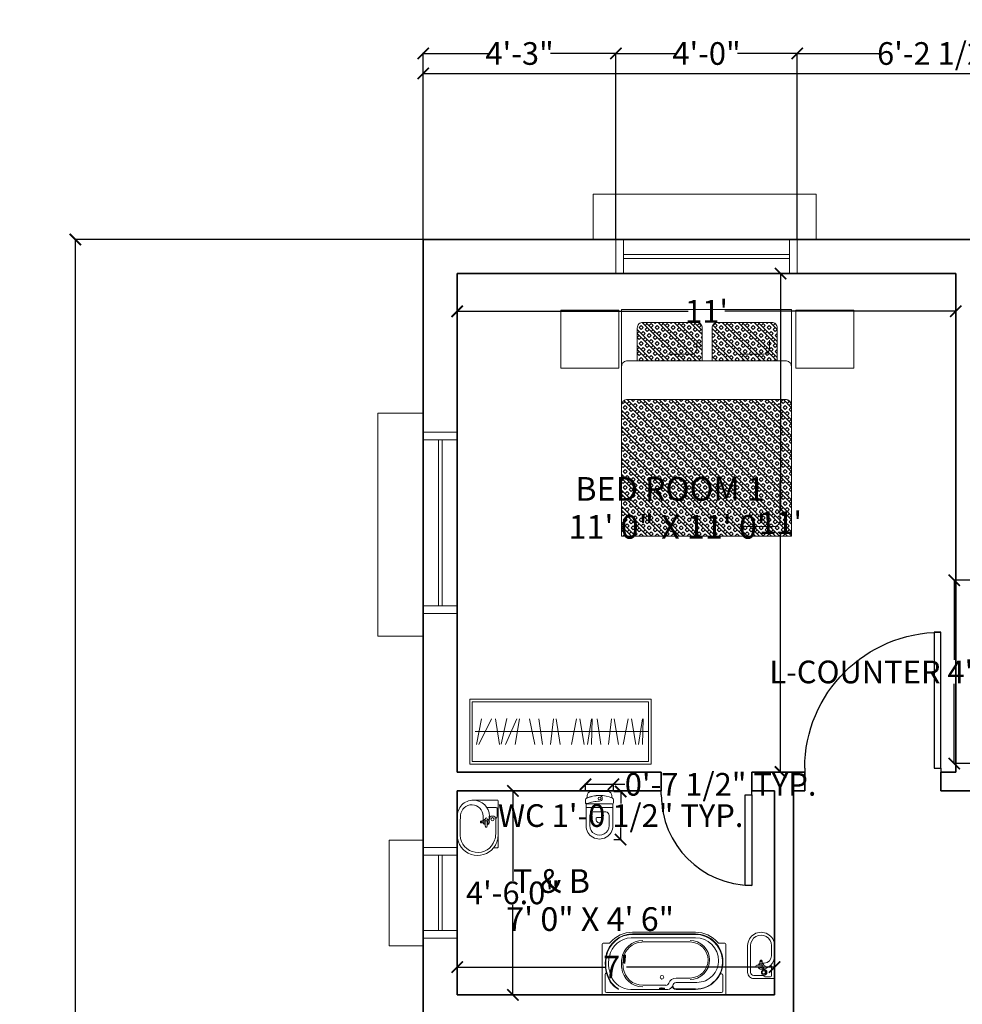
# Model space of a CAD drawing. Units: inches. Extents: x 844 to 2234, y 346 to 1084.
# Tile 3 of 93: x 844 to 1093, y 823 to 1084. Entities that reach past the tile are written whole.
import ezdxf

# ---------------------------------------------------------------- set-up
doc = ezdxf.new("R2010")
doc.units = ezdxf.units.IN
doc.header["$MEASUREMENT"] = 0
for name, color, linetype, lineweight in [('A-ANNO-DIMS', 2, 'Continuous', 18), ('A-AREA-IDEN', 7, 'Continuous', 18), ('A-FLOR-FIXT', 8, 'Continuous', 18), ('A-WALL', 7, 'Continuous', 35), ('beds', 130, 'Continuous', 18), ('doors', 170, 'Continuous', 25), ('furniture', 8, 'Continuous', 18), ('windows', 1, 'Continuous', 18)]:
    doc.layers.add(name, color=color, linetype=linetype, lineweight=lineweight)
doc.styles.get("Standard").update_dxf_attribs({"font": 'arial.ttf'})
doc.dimstyles.get("Standard").update_dxf_attribs({"dimtxt": 6, "dimasz": 3, "dimexe": 0.18, "dimexo": 0.0625, "dimgap": 0.09, "dimtad": 0, "dimtih": 1, "dimtoh": 1, "dimdec": 1, "dimzin": 0, "dimdsep": 46, "dimlunit": 3, "dimtxsty": 'Standard', "dimblk": 'ARCHTICK', "dimcen": 0.09, "dimadec": 0, "dimazin": 0, "dimtfac": 1, "dimtdec": 1, "dimtofl": 0, "dimtmove": 0, "dimatfit": 3, "dimfxl": 1, "dimtolj": 1, "dimtzin": 0, "dimarcsym": 0})
pattern_1 = [(135, (-1377.70473, -125.71507), (-0.070710678, -0.070710678), []), (135, (-1377.68705, -125.69739), (-0.070710678, -0.070710678), []), (45, (-1377.70473, -125.71507), (-0.070710678, 0.070710678), [-0.025, 0.025]), (45, (-1377.72241, -125.69739), (-0.070710678, 0.070710678), [-0.025, 0.025]), (45, (-1377.74009, -125.67972), (-0.070710678, 0.070710678), [0.025, -0.025]), (45, (-1377.75776, -125.66204), (-0.070710678, 0.070710678), [0.025, -0.025]), (135, (-1377.66938, -125.67972), (-0.070710678, -0.070710678), [0.025, -0.025]), (135, (-1377.6517, -125.66204), (-0.070710678, -0.070710678), [0.025, -0.025])]

# ---------------------------------------------------------------- blocks, each defined once
blk = doc.blocks.new('*U2')
for p, q in [((0, 0), (0, -6)), ((36, 0), (36, -6))]:
    blk.add_line(p, q)
blk.add_lwpolyline([(0, 0), (0, 36), (1.75, 36), (1.75, 0)], close=True)
blk.add_arc((0, 0), 36, 0, 90)
blk = doc.blocks.new('*U4')
for p, q in [((0, 0), (0, -6)), ((24, 0), (24, -6))]:
    blk.add_line(p, q)
blk.add_lwpolyline([(0, 0), (0, 24), (1.75, 24), (1.75, 0)], close=True)
blk.add_arc((0, 0), 24, 0, 90)
blk = doc.blocks.new('MAT-P10')
h = blk.add_hatch()
h.set_pattern_fill('BOX', color=256, scale=0.1, angle=45, style=0)
h.set_pattern_definition(pattern_1)
h.paths.add_polyline_path([(-0.1565, 1.4605), (0.417, 1.4605), (0.417, 1.7513, 0.414214), (0.367, 1.8013), (-0.1065, 1.8013, 0.414214), (-0.1565, 1.7513)])
h.paths.add_polyline_path([(0.5052, 1.4604), (1.0792, 1.4604), (1.0792, 1.7513, 0.414214), (1.0292, 1.8013), (0.5552, 1.8013, 0.414214), (0.5052, 1.7513)])
h = blk.add_hatch()
h.set_pattern_fill('BOX', color=256, scale=0.1, angle=45, style=0)
h.set_pattern_definition(pattern_1)
edge = h.paths.add_edge_path()
edge.add_line((1.2049, -0.085), (1.2049, 1.0625))
edge.add_ellipse((1.1608, 1.0627), major_axis=(0, 0.0568), ratio=0.776379, start_angle=270, end_angle=360)
edge.add_line((1.1608, 1.1195), (-0.251, 1.1195))
edge.add_ellipse((-0.251, 1.0627), major_axis=(0, 0.0568), ratio=0.776379, start_angle=0, end_angle=88.13958)
edge.add_line((-0.2951, 1.0641), (-0.2951, -0.085))
edge.add_line((-0.2951, -0.085), (1.2049, -0.085))
for p, q in [((-0.251, 1.4605), (1.1608, 1.4604)), ((-0.251, 1.1195), (1.1608, 1.1195)), ((1.1017, 0.406), (1.1017, 0.0572)), ((1.0576, 0.0004), (0.7754, 0.0004))]:
    blk.add_line(p, q)
for points in [[(1.2049, -0.085), (-0.2951, -0.085), (-0.2951, 1.9151), (1.2049, 1.915)], [(-0.8301, 1.9091), (-0.3191, 1.9091), (-0.3191, 1.3981), (-0.8301, 1.3981)], [(1.2441, 1.9091), (1.755, 1.9091), (1.755, 1.3981), (1.2441, 1.3981)]]:
    blk.add_lwpolyline(points, close=True)
for points in [[(0.417, 1.4604), (0.417, 1.7513, 0.414214), (0.367, 1.8013), (-0.1065, 1.8013, 0.414214), (-0.1565, 1.7513), (-0.1565, 1.4604)], [(1.0792, 1.4603), (1.0792, 1.7513, 0.414214), (1.0292, 1.8013), (0.5552, 1.8013, 0.414214), (0.5052, 1.7513), (0.5052, 1.4604)], [(0.3702, 1.6242), (0.3702, 1.5715, -0.414214), (0.3202, 1.5215), (0.1113, 1.5215)], [(1.0117, 1.6438), (1.0117, 1.5715, -0.414214), (0.9617, 1.5215), (0.7528, 1.5215)]]:
    blk.add_lwpolyline(points, format="xyb")
at = {"extrusion": (0, 0, -1)}
for centre, start_param, end_param in [((-0.251, 1.4036), 4.712389, 6.283185), ((1.1608, 1.4036), 0, 1.570796), ((-0.251, 1.0627), 4.712389, 6.283185), ((1.1608, 1.0627), 0, 1.570796), ((1.0576, 0.0572), 1.570796, 3.141593), ((1.0576, 0.0572), 1.570796, 3.141593)]:
    blk.add_ellipse(centre, major_axis=(0, 0.0568), ratio=0.776379, start_param=start_param, end_param=end_param, dxfattribs=at)
blk = doc.blocks.new('A$C7A17768A')
for p, q in [((-2.8, 0), (0, 0)), ((-2.8, -1), (-2.8, 0)), ((0, -1), (0, 0)), ((-2.76, -0.04), (-0.04, -0.04)), ((-2.76, -0.96), (-2.76, -0.04)), ((-0.04, -0.96), (-0.04, -0.04)), ((-2.617, -0.3), (-2.694, -0.7)), ((-2.66, -0.7), (-2.466, -0.3)), ((-2.403, -0.3), (-2.342, -0.7)), ((-2.229, -0.296), (-2.317, -0.696)), ((-2.074, -0.3), (-2.25, -0.7)), ((-2.096, -0.7), (-2.033, -0.3)), ((-1.875, -0.3), (-1.796, -0.7)), ((-1.732, -0.3), (-1.675, -0.7)), ((-1.555, -0.7), (-1.507, -0.3)), ((-1.467, -0.3), (-1.403, -0.7)), ((-1.227, -0.7), (-1.151, -0.3)), ((-1.098, -0.3), (-1.034, -0.7)), ((-0.98, -0.7), (-0.921, -0.3)), ((-0.908, -0.3), (-0.919, -0.7)), ((-0.834, -0.3), (-0.777, -0.7)), ((-0.657, -0.7), (-0.61, -0.3)), ((-0.57, -0.3), (-0.505, -0.7)), ((-0.429, -0.7), (-0.353, -0.3)), ((-0.301, -0.3), (-0.237, -0.7)), ((-0.192, -0.7), (-0.133, -0.3)), ((-0.12, -0.3), (-0.131, -0.7)), ((-0.04, -0.5), (-2.716, -0.5)), ((-2.8, -1), (0, -1)), ((-2.76, -0.96), (-0.04, -0.96))]:
    blk.add_line(p, q)
blk = doc.blocks.new('2SABICO')
at = {"color": 0, "linetype": 'ByBlock'}
for p, q in [((0.478, 0.195), (0.089, 0.195)), ((0.478, 0.152), (0.089, 0.152)), ((0, 0.106), (0, 0)), ((0, 0), (0, -0.18)), ((0.043, -0.039), (0.043, 0.106)), ((0.135, 0), (0.135, -0.003)), ((0.168, 0.064), (0.168, -0.015)), ((0.192, 0.064), (0.192, -0.015)), ((0.221, 0.012), (0.222, 0.012)), ((0.223, 0.016), (0.223, -0.016)), ((0.224, 0.017), (0.245, 0.017)), ((0.246, 0.016), (0.246, -0.016)), ((0.25, 0.014), (0.246, 0.014)), ((0.26, 0.01), (0.268, 0.01)), ((0.268, -0.01), (0.268, 0.01)), ((0.268, 0.01), (0.269, 0.009)), ((0.269, -0.009), (0.269, 0.009)), ((0.023, -0.057), (0.023, -0.135)), ((0.135, 0), (0.135, -0.039)), ((0.168, -0.015), (0.192, -0.015)), ((0.168, -0.015), (0.168, -0.046)), ((0.192, -0.015), (0.192, -0.046)), ((0.221, -0.012), (0.222, -0.012)), ((0.224, -0.017), (0.245, -0.017)), ((0.225, -0.017), (0.225, -0.047)), ((0.25, -0.014), (0.246, -0.014)), ((0.26, -0.01), (0.268, -0.01)), ((0.268, -0.01), (0.269, -0.009)), ((0.015, -0.195), (0.478, -0.195)), ((0.038, -0.15), (0.179, -0.15)), ((0.33, -0.152), (0.478, -0.152))]:
    blk.add_line(p, q, dxfattribs=at)
for radius in [0.035, 0.023]:
    blk.add_circle((0.089, -0.039), radius, dxfattribs=at)
for centre, radius, start, end in [((0.089, 0.106), 0.089, 90, 180), ((0.089, 0.106), 0.046, 90, 180), ((0.478, 0), 0.195, 270, 90), ((0.478, 0), 0.152, 270, 90), ((0.18, 0), 0.045, 105.6643, 180), ((0.18, 0), 0.042, 106.8152, 252.6853), ((0.18, 0), 0.0235, 121.1327, 237.8651), ((0.18, 0.064), 0.0121, 0, 180), ((0.18, 0), 0.045, 17.0576, 74.3357), ((0.18, 0), 0.042, 287.3147, 73.1848), ((0.18, 0), 0.0235, 302.1349, 58.8673), ((0.221, 0.013), 0.001, 197.9471, 270), ((0.222, 0.013), 0.001, 270, 0), ((0.224, 0.016), 0.001, 90, 180), ((0.245, 0.016), 0.001, 0, 90), ((0.25, 0), 0.0143, 270, 90), ((0.041, -0.057), 0.018, 99.5941, 180), ((0.038, -0.135), 0.015, 180, 270), ((0.037, -0.033), 0.006, 279.5941, 0), ((0.089, -0.039), 0.046, 180, 360), ((0.326, -0.003), 0.191, 180, 270), ((0.18, -0.046), 0.0125, 180, 0), ((0.179, -0.14), 0.01, 270, 42.9682), ((0.221, -0.013), 0.001, 90, 162.0529), ((0.222, -0.013), 0.001, 0, 90), ((0.224, -0.016), 0.001, 180, 270), ((0.33, -0.047), 0.105, 180, 270), ((0.245, -0.016), 0.001, 270, 0), ((0.015, -0.18), 0.015, 180, 270)]:
    blk.add_arc(centre, radius, start, end, dxfattribs=at)
blk = doc.blocks.new('2SAINCO')
at = {"color": 0, "linetype": 'ByBlock'}
for p, q in [((0.06, 0.181), (0.085, 0.181)), ((0.114, 0.203), (0.165, 0.203)), ((0.496, 0.195), (0.178, 0.195)), ((0.18, -0.188), (0.18, 0.188)), ((0.231, 0.185), (0.231, -0.185)), ((0.234, 0.185), (0.234, -0.185)), ((0, -0.121), (0, 0.121)), ((0.496, 0.14), (0.347, 0.14)), ((0.394, 0.05), (0.407, 0.05)), ((0.496, -0.14), (0.347, -0.14)), ((0.394, -0.05), (0.407, -0.05)), ((0.06, -0.181), (0.085, -0.181)), ((0.114, -0.201), (0.165, -0.201)), ((0.114, -0.203), (0.165, -0.203)), ((0.496, -0.195), (0.178, -0.195))]:
    blk.add_line(p, q, dxfattribs=at)
blk.add_circle((0.1, 0), 0.02, dxfattribs=at)
for centre, radius, start, end in [((0.06, 0.121), 0.06, 90, 180), ((0.517, 0), 0.46, 155.909, 204.091), ((0.085, 0.196), 0.015, 270, 344.534), ((0.114, 0.188), 0.015, 90, 164.534), ((0.165, 0.188), 0.015, 0, 90), ((0.221, 0.185), 0.01, 0, 90), ((0.224, 0.185), 0.01, 0, 90), ((0.496, 0), 0.195, 270, 90), ((0.1, 0), 0.0405, 360, 180), ((0.517, 0), 0.458, 180, 204.67), ((0.66, 0.008), 0.52, 180.891, 201.3823), ((2.295, 0), 2, 177.3546, 182.6454), ((0.347, 0.09), 0.05, 90, 177.3546), ((0.677, 0), 0.3, 172.9459, 187.0541), ((0.394, 0.035), 0.015, 90, 172.9459), ((0.407, 0), 0.05, 270, 90), ((0.496, 0), 0.14, 270, 90), ((0.06, -0.121), 0.06, 180, 270), ((0.347, -0.09), 0.05, 182.6454, 270), ((0.394, -0.035), 0.015, 187.0541, 270), ((0.085, -0.196), 0.015, 15.466, 90), ((0.114, -0.188), 0.015, 195.466, 270), ((0.114, -0.188), 0.013, 195.466, 270), ((0.165, -0.188), 0.013, 270, 30), ((0.165, -0.188), 0.015, 270, 0), ((0.221, -0.185), 0.01, 270, 0), ((0.224, -0.185), 0.01, 270, 0)]:
    blk.add_arc(centre, radius, start, end, dxfattribs=at)
blk = doc.blocks.new('2SABACO')
at = {"color": 0}
for p, q in [((1.341, 0.91), (0.429, 0.91)), ((1.341, 0.885), (0.429, 0.885)), ((1.341, 0.879), (0.429, 0.879)), ((-0.015, 0.735), (-0.015, 0.015)), ((0, 0.75), (0.08, 0.75)), ((1.341, 0.831), (0.407, 0.831)), ((1.263, 0.769), (0.562, 0.769)), ((1.77, 0.75), (1.69, 0.75)), ((1.785, 0.015), (1.785, 0.735)), ((0.03, 0.302), (0.03, 0.053)), ((1.263, 0.245), (1.06, 0.245)), ((1.363, 0.181), (1.06, 0.181)), ((1.74, 0.053), (1.74, 0.286)), ((0, 0), (1.77, 0)), ((0.048, 0.035), (1.722, 0.035)), ((0.401, 0.08), (0.942, 0.08)), ((0.578, 0.139), (0.911, 0.139)), ((1.343, 0.086), (1.06, 0.086)), ((1.343, 0.079), (1.06, 0.079))]:
    blk.add_line(p, q, dxfattribs=at)
blk.add_circle((0.855, 0.256), 0.026, dxfattribs=at)
for centre, radius, start, end in [((0.428, 0.49), 0.395, 98.9726, 181.1954), ((0.428, 0.49), 0.389, 98.9726, 181.2301), ((0.429, 0.48), 0.43, 90, 139.2943), ((0.429, 0.48), 0.405, 90, 98.9726), ((0.429, 0.48), 0.399, 90, 98.9726), ((1.341, 0.48), 0.43, 40.7057, 90), ((1.341, 0.485), 0.401, 359.4627, 90), ((1.341, 0.485), 0.394, 3.5237, 90), ((0, 0.735), 0.015, 90, 180), ((0.08, 0.78), 0.03, 270, 319.2943), ((0.425, 0.49), 0.342, 93.1008, 168.0202), ((0.578, 0.481), 0.311, 90, 172.609), ((0.578, 0.481), 0.288, 93.3767, 172.609), ((1.263, 0.507), 0.285, 270, 90), ((1.263, 0.507), 0.262, 270, 90), ((1.341, 0.495), 0.336, 0, 90), ((1.69, 0.78), 0.03, 220.7057, 270), ((1.77, 0.735), 0.015, 0, 90), ((0.559, 0.454), 0.48, 163.1286, 202.3619), ((0.559, 0.454), 0.528, 177.0415, 202.3619), ((0.559, 0.454), 0.521, 177.0156, 202.3619), ((0.79, 0.454), 0.525, 172.609, 180), ((0.79, 0.454), 0.525, 180, 187.391), ((0.79, 0.454), 0.502, 172.609, 180), ((0.79, 0.454), 0.502, 180, 187.391), ((1.343, 0.477), 0.392, 270, 4.5675), ((1.343, 0.477), 0.398, 270, 0.539), ((1.363, 0.495), 0.314, 270, 2.2815), ((0.042, 0.302), 0.0116, 16.3184, 180.0001), ((0.578, 0.427), 0.311, 187.391, 270), ((0.578, 0.427), 0.288, 187.391, 270), ((1.718, 0.286), 0.0222, 0, 152.9966), ((0.401, 0.389), 0.357, 202.3619, 239.8287), ((0.401, 0.389), 0.351, 202.3619, 239.2093), ((0.401, 0.389), 0.309, 202.3619, 270), ((0.911, 0.183), 0.045, 270, 341.2369), ((1.06, 0.133), 0.112, 90, 161.2369), ((1.06, 0.133), 0.0475, 90, 270), ((0, 0.015), 0.015, 180, 270), ((0.048, 0.053), 0.018, 180, 270), ((0.559, 0.454), 0.48, 250.7818, 251.0555), ((0.821, 0.092), 0.00282, 119.7759, 180), ((0.821, 0.092), 0.00282, 180, 240.2241), ((0.837, 0.064), 0.0347, 103.3326, 119.7759), ((0.835, 0.025), 0.071, 96.5949, 102.1924), ((0.837, 0.12), 0.0347, 240.2241, 256.6674), ((0.847, -0.08), 0.177, 92.7417, 96.5949), ((0.848, 0.02), 0.0808, 95.6065, 103.3326), ((0.848, 0.164), 0.0808, 256.6674, 264.3935), ((0.855, -0.252), 0.349, 90, 92.7417), ((0.855, -0.053), 0.153, 90, 95.6065), ((0.855, 0.237), 0.153, 264.3935, 270), ((0.855, -0.053), 0.153, 84.3935, 90), ((0.855, -0.252), 0.349, 87.2583, 90), ((0.855, 0.237), 0.153, 270, 275.6065), ((0.862, 0.02), 0.0808, 76.6674, 84.3935), ((0.862, 0.164), 0.0808, 275.6065, 283.3326), ((0.863, -0.08), 0.177, 83.4051, 87.2583), ((0.873, 0.064), 0.0347, 60.2241, 76.6674), ((0.873, 0.12), 0.0347, 283.3326, 299.7759), ((0.875, 0.025), 0.071, 77.8076, 83.4051), ((0.889, 0.092), 0.00282, 360, 60.2241), ((0.889, 0.092), 0.00282, 299.7759, 360), ((0.942, 0.145), 0.065, 270, 349.4977), ((1.06, 0.133), 0.054, 180, 270), ((1.722, 0.053), 0.018, 270, 0), ((1.77, 0.015), 0.015, 270, 0)]:
    blk.add_arc(centre, radius, start, end, dxfattribs=at)
blk = doc.blocks.new('2SALACO2')
at = {"color": 0}
for p, q in [((0, 0), (-0.392, 0)), ((0.28, 0), (0, 0)), ((-0.402, -0.01), (-0.402, -0.36)), ((-0.293, -0.026), (-0.293, -0.15)), ((-0.283, -0.016), (-0.166, -0.016)), ((-0.169, -0.128), (-0.085, -0.128)), ((-0.112, -0.035), (-0.133, -0.035)), ((-0.124, -0.035), (0.09, -0.035)), ((0.29, -0.01), (0.29, -0.064)), ((-0.102, -0.219), (-0.169, -0.219)), ((-0.1, -0.161), (-0.131, -0.161)), ((-0.1, -0.186), (-0.131, -0.186)), ((-0.102, -0.217), (-0.102, -0.234)), ((-0.07, -0.216), (-0.101, -0.216)), ((-0.07, -0.235), (-0.101, -0.235)), ((-0.1, -0.161), (-0.1, -0.186)), ((-0.021, -0.161), (-0.1, -0.161)), ((-0.021, -0.186), (-0.1, -0.186)), ((-0.098, -0.214), (-0.098, -0.216)), ((-0.097, -0.239), (-0.098, -0.241)), ((-0.098, -0.241), (-0.098, -0.248)), ((-0.098, -0.241), (-0.073, -0.241)), ((-0.073, -0.248), (-0.098, -0.248)), ((-0.097, -0.235), (-0.097, -0.239)), ((-0.074, -0.239), (-0.097, -0.239)), ((-0.097, -0.248), (-0.097, -0.256)), ((-0.073, -0.256), (-0.097, -0.256)), ((-0.097, -0.256), (-0.094, -0.257)), ((-0.077, -0.257), (-0.094, -0.257)), ((-0.073, -0.256), (-0.077, -0.257)), ((-0.074, -0.235), (-0.074, -0.239)), ((-0.074, -0.239), (-0.073, -0.241)), ((-0.073, -0.214), (-0.073, -0.216)), ((-0.073, -0.241), (-0.073, -0.248)), ((-0.073, -0.248), (-0.073, -0.256)), ((-0.069, -0.217), (-0.069, -0.234))]:
    blk.add_line(p, q, dxfattribs=at)
blk.add_lwpolyline([(-0.402, -0.36, 0.423787), (-0.161, -0.593, 0.423787)], format="xyb", dxfattribs=at)
blk.add_circle((-0.124, -0.081), 0.023, dxfattribs=at)
for centre, radius, start, end in [((-0.392, -0.01), 0.01, 90, 180), ((0.28, -0.01), 0.01, 0, 90), ((-0.169, -0.36), 0.233, 90, 180), ((-0.283, -0.026), 0.01, 90, 180), ((-0.124, -0.081), 0.0462, 90, 270), ((-0.166, -0.046), 0.03, 31.2573, 90), ((-0.133, -0.026), 0.009, 211.2573, 270), ((-0.085, -0.173), 0.042, 16.8152, 162.6853), ((-0.085, -0.173), 0.0458, 15.3964, 90), ((0.09, -0.29), 0.255, 68.9449, 90), ((0.105, -0.295), 0.255, 271.0077, 72.4499), ((0.105, -0.297), 0.297, 271.4871, 51.4524), ((0.105, -0.297), 0.297, 51.4524, 87.1707), ((-0.169, -0.383), 0.164, 90, 265.4963), ((-0.285, -0.15), 0.008, 180, 299.1062), ((-0.131, -0.173), 0.0125, 90, 270), ((-0.085, -0.173), 0.042, 197.3147, 343.1848), ((-0.085, -0.173), 0.0235, 31.1327, 147.8651), ((-0.085, -0.173), 0.0235, 212.1349, 328.8673), ((-0.101, -0.217), 0.001, 90, 180), ((-0.101, -0.234), 0.001, 180, 270), ((-0.085, -0.173), 0.0458, 289.9182, 344.6036), ((-0.07, -0.217), 0.001, 0, 90), ((-0.07, -0.234), 0.001, 270, 0), ((-0.021, -0.173), 0.0121, 270, 90), ((0.021, 4.449), 5, 267.6742, 271.0081), ((-0.017, 4.405), 5, 268.3511, 271.4874)]:
    blk.add_arc(centre, radius, start, end, dxfattribs=at)
blk = doc.blocks.new('_ArchTick')
at = {"color": 0, "linetype": 'ByBlock', "const_width": 0.15}
blk.add_lwpolyline([(-0.5, -0.5), (0.5, 0.5)], dxfattribs=at)
blk = doc.blocks.new('*D23')
at = {"layer": 'A-ANNO-DIMS', "color": 0, "lineweight": -2, "transparency": 16777216}
for p, q in [((1055.36, 1016.31), (1045.04, 1016.31)), ((1045.22, 1016.31), (1045.22, 953.41)), ((1045.22, 884.31), (1045.22, 947.21)), ((1044.68, 884.31), (1045.4, 884.31))]:
    blk.add_line(p, q, dxfattribs=at)
at = {"layer": 'Defpoints', "color": 0, "transparency": 16777216}
for p in [(1055.42, 1016.31), (1044.62, 884.31), (1045.22, 884.31)]:
    blk.add_point(p, dxfattribs=at)
at = {"layer": 'A-ANNO-DIMS', "color": 0, "lineweight": -2, "transparency": 16777216, "xscale": 3, "yscale": 3, "zscale": 3}
for p, rotation in [((1045.22, 1016.31), 90), ((1045.22, 884.31), 270)]:
    blk.add_blockref('_ArchTick', p, dxfattribs=dict(at, rotation=rotation))
at = {"layer": 'A-ANNO-DIMS', "color": 0, "transparency": 16777216, "insert": (1045.22, 950.31), "char_height": 6, "attachment_point": 5}
blk.add_mtext("\\A1;11'", dxfattribs=at)
blk = doc.blocks.new('*D24')
at = {"layer": 'A-ANNO-DIMS', "color": 0, "lineweight": -2, "transparency": 16777216}
for p, q in [((959.62, 1008.78), (959.62, 1006.13)), ((959.62, 1006.31), (1020.72, 1006.31)), ((1091.62, 1006.31), (1030.51, 1006.31)), ((1091.62, 1008.78), (1091.62, 1006.13))]:
    blk.add_line(p, q, dxfattribs=at)
at = {"layer": 'Defpoints', "color": 0, "transparency": 16777216}
for p in [(959.62, 1008.84), (1091.62, 1008.84), (1091.62, 1006.31)]:
    blk.add_point(p, dxfattribs=at)
at = {"layer": 'A-ANNO-DIMS', "color": 0, "lineweight": -2, "transparency": 16777216, "xscale": 3, "yscale": 3, "zscale": 3, "rotation": 180}
blk.add_blockref('_ArchTick', (959.62, 1006.31), dxfattribs=at)
at = {"layer": 'A-ANNO-DIMS', "color": 0, "lineweight": -2, "transparency": 16777216, "xscale": 3, "yscale": 3, "zscale": 3}
blk.add_blockref('_ArchTick', (1091.62, 1006.31), dxfattribs=at)
at = {"layer": 'A-ANNO-DIMS', "color": 0, "transparency": 16777216, "insert": (1025.62, 1006.31), "char_height": 6, "attachment_point": 5}
blk.add_mtext("\\A1;11'", dxfattribs=at)
blk = doc.blocks.new('*D39')
at = {"layer": 'A-ANNO-DIMS', "color": 0, "lineweight": -2, "transparency": 16777216}
for p, q in [((959.62, 827.5), (959.62, 832.84)), ((959.62, 832.66), (998.79, 832.66)), ((1043.62, 832.66), (1004.44, 832.66)), ((1043.62, 827.5), (1043.62, 832.84))]:
    blk.add_line(p, q, dxfattribs=at)
at = {"layer": 'Defpoints', "color": 0, "transparency": 16777216}
for p in [(959.62, 832.66), (959.62, 827.44), (1043.62, 827.44)]:
    blk.add_point(p, dxfattribs=at)
at = {"layer": 'A-ANNO-DIMS', "color": 0, "lineweight": -2, "transparency": 16777216, "xscale": 3, "yscale": 3, "zscale": 3, "rotation": 180}
blk.add_blockref('_ArchTick', (959.62, 832.66), dxfattribs=at)
at = {"layer": 'A-ANNO-DIMS', "color": 0, "lineweight": -2, "transparency": 16777216, "xscale": 3, "yscale": 3, "zscale": 3}
blk.add_blockref('_ArchTick', (1043.62, 832.66), dxfattribs=at)
at = {"layer": 'A-ANNO-DIMS', "color": 0, "transparency": 16777216, "insert": (1001.62, 832.66), "char_height": 6, "attachment_point": 5}
blk.add_mtext("\\A1;7'", dxfattribs=at)
blk = doc.blocks.new('*D40')
at = {"layer": 'A-ANNO-DIMS', "color": 0, "lineweight": -2, "transparency": 16777216}
for p, q in [((975.39, 879.31), (974.2, 879.31)), ((974.38, 879.31), (974.38, 855.46)), ((974.38, 825.31), (974.38, 849.16)), ((975.39, 825.31), (974.2, 825.31))]:
    blk.add_line(p, q, dxfattribs=at)
at = {"layer": 'Defpoints', "color": 0, "transparency": 16777216}
for p in [(975.46, 879.31), (974.38, 825.31), (975.46, 825.31)]:
    blk.add_point(p, dxfattribs=at)
at = {"layer": 'A-ANNO-DIMS', "color": 0, "lineweight": -2, "transparency": 16777216, "xscale": 3, "yscale": 3, "zscale": 3}
for p, rotation in [((974.38, 879.31), 90), ((974.38, 825.31), 270)]:
    blk.add_blockref('_ArchTick', p, dxfattribs=dict(at, rotation=rotation))
at = {"layer": 'A-ANNO-DIMS', "color": 0, "transparency": 16777216, "insert": (974.38, 852.31), "char_height": 6, "attachment_point": 5}
blk.add_mtext('\\A1;4\'-6.0"', dxfattribs=at)
blk = doc.blocks.new('*D55')
at = {"layer": 'A-ANNO-DIMS', "color": 0, "lineweight": -2, "transparency": 16777216}
for p, q in [((950.62, 1025.37), (950.62, 1069.43)), ((950.62, 1069.25), (1173.9, 1069.25)), ((1429.62, 1069.25), (1206.34, 1069.25)), ((1429.62, 1025.37), (1429.62, 1069.43))]:
    blk.add_line(p, q, dxfattribs=at)
at = {"layer": 'Defpoints', "color": 0, "transparency": 16777216}
for p in [(1429.62, 1069.25), (950.62, 1025.31), (1429.62, 1025.31)]:
    blk.add_point(p, dxfattribs=at)
at = {"layer": 'A-ANNO-DIMS', "color": 0, "lineweight": -2, "transparency": 16777216, "xscale": 3, "yscale": 3, "zscale": 3, "rotation": 180}
blk.add_blockref('_ArchTick', (950.62, 1069.25), dxfattribs=at)
at = {"layer": 'A-ANNO-DIMS', "color": 0, "lineweight": -2, "transparency": 16777216, "xscale": 3, "yscale": 3, "zscale": 3}
blk.add_blockref('_ArchTick', (1429.62, 1069.25), dxfattribs=at)
at = {"layer": 'A-ANNO-DIMS', "color": 0, "transparency": 16777216, "insert": (1190.12, 1069.25), "char_height": 6, "attachment_point": 5}
blk.add_mtext('\\A1;39\'-11.0"', dxfattribs=at)
blk = doc.blocks.new('*D56')
at = {"layer": 'A-ANNO-DIMS', "color": 0, "lineweight": -2, "transparency": 16777216}
for p, q in [((950.55, 1025.31), (858.33, 1025.31)), ((858.51, 1025.31), (858.51, 730.96)), ((858.51, 430.31), (858.51, 724.66)), ((950.55, 430.31), (858.33, 430.31))]:
    blk.add_line(p, q, dxfattribs=at)
at = {"layer": 'Defpoints', "color": 0, "transparency": 16777216}
for p in [(950.62, 1025.31), (858.51, 430.31), (950.62, 430.31)]:
    blk.add_point(p, dxfattribs=at)
at = {"layer": 'A-ANNO-DIMS', "color": 0, "lineweight": -2, "transparency": 16777216, "xscale": 3, "yscale": 3, "zscale": 3}
for p, rotation in [((858.51, 1025.31), 90), ((858.51, 430.31), 270)]:
    blk.add_blockref('_ArchTick', p, dxfattribs=dict(at, rotation=rotation))
at = {"layer": 'A-ANNO-DIMS', "color": 0, "transparency": 16777216, "insert": (858.51, 727.81), "char_height": 6, "attachment_point": 5}
blk.add_mtext('\\A1;49\'-7.0"', dxfattribs=at)
blk = doc.blocks.new('WIN-48IN')
for p, q in [((0, 9), (0, 21)), ((0, 21), (59, 21)), ((59, 9), (59, 21)), ((6, 9), (0, 9)), ((54, 9), (6, 9)), ((6, 9), (6, 0)), ((8, 9), (8, 0)), ((52, 0), (52, 9)), ((54, 0), (54, 9)), ((54, 9), (59, 9)), ((8, 5), (52, 5)), ((8, 4), (52, 4)), ((6, 0), (54, 0))]:
    blk.add_line(p, q)
blk = doc.blocks.new('WIN-24IN')
for p, q in [((9, 28), (0, 28)), ((0, 0), (0, 28)), ((9, 26), (9, 28)), ((18, 26), (9, 26)), ((9, 26), (9, 2)), ((18, 24), (9, 24)), ((13, 4), (13, 24)), ((14, 4), (14, 24)), ((18, 2), (18, 26)), ((9, 4), (18, 4)), ((9, 2), (18, 2)), ((9, 2), (9, 0)), ((9, 0), (0, 0))]:
    blk.add_line(p, q)
blk = doc.blocks.new('*D113')
at = {"layer": 'A-ANNO-DIMS', "color": 0, "lineweight": -2, "transparency": 16777216}
for p, q in [((1001.04, 879.15), (1003.07, 879.15)), ((1002.89, 879.15), (1002.89, 875.97)), ((1002.89, 866.41), (1002.89, 869.59)), ((1001.04, 866.41), (1003.07, 866.41))]:
    blk.add_line(p, q, dxfattribs=at)
at = {"layer": 'Defpoints', "color": 0, "transparency": 16777216}
for p in [(1000.98, 879.15), (1000.98, 866.41), (1002.89, 866.41)]:
    blk.add_point(p, dxfattribs=at)
at = {"layer": 'A-ANNO-DIMS', "color": 0, "lineweight": -2, "transparency": 16777216, "xscale": 3, "yscale": 3, "zscale": 3}
for p, rotation in [((1002.89, 879.15), 90), ((1002.89, 866.41), 270)]:
    blk.add_blockref('_ArchTick', p, dxfattribs=dict(at, rotation=rotation))
at = {"layer": 'A-ANNO-DIMS', "color": 0, "transparency": 16777216, "insert": (1002.89, 872.78), "char_height": 6, "attachment_point": 5}
blk.add_mtext('\\A1;WC 1\'-0 1/2" TYP.', dxfattribs=at)
blk = doc.blocks.new('*D114')
at = {"layer": 'A-ANNO-DIMS', "color": 0, "lineweight": -2, "transparency": 16777216}
for p, q in [((993.58, 879.21), (993.58, 881.24)), ((1000.98, 879.21), (1000.98, 881.24)), ((993.58, 881.06), (1000.98, 881.06)), ((1000.98, 881.06), (1003.98, 881.06))]:
    blk.add_line(p, q, dxfattribs=at)
at = {"layer": 'Defpoints', "color": 0, "transparency": 16777216}
for p in [(993.58, 879.15), (1000.98, 881.06), (1000.98, 879.15)]:
    blk.add_point(p, dxfattribs=at)
at = {"layer": 'A-ANNO-DIMS', "color": 0, "lineweight": -2, "transparency": 16777216, "xscale": 3, "yscale": 3, "zscale": 3, "rotation": 180}
blk.add_blockref('_ArchTick', (993.58, 881.06), dxfattribs=at)
at = {"layer": 'A-ANNO-DIMS', "color": 0, "lineweight": -2, "transparency": 16777216, "xscale": 3, "yscale": 3, "zscale": 3}
blk.add_blockref('_ArchTick', (1000.98, 881.06), dxfattribs=at)
at = {"layer": 'A-ANNO-DIMS', "color": 0, "transparency": 16777216, "insert": (1029.35, 881.06), "char_height": 6, "attachment_point": 5}
blk.add_mtext('\\A1;0\'-7 1/2" TYP.', dxfattribs=at)
blk = doc.blocks.new('*D131')
at = {"layer": 'A-ANNO-DIMS', "color": 0, "lineweight": -2, "transparency": 16777216}
for p, q in [((1098.42, 935.09), (1091.02, 935.09)), ((1091.2, 935.09), (1091.2, 914)), ((1091.2, 886.53), (1091.2, 907.62)), ((1098.42, 886.53), (1091.02, 886.53))]:
    blk.add_line(p, q, dxfattribs=at)
at = {"layer": 'Defpoints', "color": 0, "transparency": 16777216}
for p in [(1091.2, 935.09), (1098.48, 935.09), (1098.48, 886.53)]:
    blk.add_point(p, dxfattribs=at)
at = {"layer": 'A-ANNO-DIMS', "color": 0, "lineweight": -2, "transparency": 16777216, "xscale": 3, "yscale": 3, "zscale": 3}
for p, rotation in [((1091.2, 935.09), 90), ((1091.2, 886.53), 270)]:
    blk.add_blockref('_ArchTick', p, dxfattribs=dict(at, rotation=rotation))
at = {"layer": 'A-ANNO-DIMS', "color": 0, "transparency": 16777216, "insert": (1091.2, 910.81), "char_height": 6, "attachment_point": 5}
blk.add_mtext('\\A1;L-COUNTER 4\'-0 1/2" TYP.', dxfattribs=at)
blk = doc.blocks.new('*D150')
at = {"layer": 'A-ANNO-DIMS', "color": 0, "lineweight": -2, "transparency": 16777216}
for p, q in [((950.62, 1025.37), (950.62, 1074.74)), ((950.62, 1074.56), (967.93, 1074.56)), ((1001.62, 1074.56), (984.3, 1074.56)), ((1001.62, 1025.37), (1001.62, 1074.74))]:
    blk.add_line(p, q, dxfattribs=at)
at = {"layer": 'Defpoints', "color": 0, "transparency": 16777216}
for p in [(1001.62, 1074.56), (950.62, 1025.31), (1001.62, 1025.31)]:
    blk.add_point(p, dxfattribs=at)
at = {"layer": 'A-ANNO-DIMS', "color": 0, "lineweight": -2, "transparency": 16777216, "xscale": 3, "yscale": 3, "zscale": 3, "rotation": 180}
blk.add_blockref('_ArchTick', (950.62, 1074.56), dxfattribs=at)
at = {"layer": 'A-ANNO-DIMS', "color": 0, "lineweight": -2, "transparency": 16777216, "xscale": 3, "yscale": 3, "zscale": 3}
blk.add_blockref('_ArchTick', (1001.62, 1074.56), dxfattribs=at)
at = {"layer": 'A-ANNO-DIMS', "color": 0, "transparency": 16777216, "insert": (976.12, 1074.56), "char_height": 6, "attachment_point": 5}
blk.add_mtext('\\A1;4\'-3"', dxfattribs=at)
blk = doc.blocks.new('*D151')
at = {"layer": 'A-ANNO-DIMS', "color": 0, "lineweight": -2, "transparency": 16777216}
for p, q in [((1001.62, 1025.37), (1001.62, 1074.74)), ((1001.62, 1074.56), (1017.43, 1074.56)), ((1049.62, 1074.56), (1033.8, 1074.56)), ((1049.62, 1025.37), (1049.62, 1074.74))]:
    blk.add_line(p, q, dxfattribs=at)
at = {"layer": 'Defpoints', "color": 0, "transparency": 16777216}
for p in [(1049.62, 1074.56), (1001.62, 1025.31), (1049.62, 1025.31)]:
    blk.add_point(p, dxfattribs=at)
at = {"layer": 'A-ANNO-DIMS', "color": 0, "lineweight": -2, "transparency": 16777216, "xscale": 3, "yscale": 3, "zscale": 3, "rotation": 180}
blk.add_blockref('_ArchTick', (1001.62, 1074.56), dxfattribs=at)
at = {"layer": 'A-ANNO-DIMS', "color": 0, "lineweight": -2, "transparency": 16777216, "xscale": 3, "yscale": 3, "zscale": 3}
blk.add_blockref('_ArchTick', (1049.62, 1074.56), dxfattribs=at)
at = {"layer": 'A-ANNO-DIMS', "color": 0, "transparency": 16777216, "insert": (1025.62, 1074.56), "char_height": 6, "attachment_point": 5}
blk.add_mtext('\\A1;4\'-0"', dxfattribs=at)
blk = doc.blocks.new('*D152')
at = {"layer": 'A-ANNO-DIMS', "color": 0, "lineweight": -2, "transparency": 16777216}
for p, q in [((1049.62, 1025.37), (1049.62, 1074.74)), ((1049.62, 1074.56), (1071.79, 1074.56)), ((1124.12, 1074.56), (1101.94, 1074.56)), ((1124.12, 1025.37), (1124.12, 1074.74))]:
    blk.add_line(p, q, dxfattribs=at)
at = {"layer": 'Defpoints', "color": 0, "transparency": 16777216}
for p in [(1124.12, 1074.56), (1049.62, 1025.31), (1124.12, 1025.31)]:
    blk.add_point(p, dxfattribs=at)
at = {"layer": 'A-ANNO-DIMS', "color": 0, "lineweight": -2, "transparency": 16777216, "xscale": 3, "yscale": 3, "zscale": 3, "rotation": 180}
blk.add_blockref('_ArchTick', (1049.62, 1074.56), dxfattribs=at)
at = {"layer": 'A-ANNO-DIMS', "color": 0, "lineweight": -2, "transparency": 16777216, "xscale": 3, "yscale": 3, "zscale": 3}
blk.add_blockref('_ArchTick', (1124.12, 1074.56), dxfattribs=at)
at = {"layer": 'A-ANNO-DIMS', "color": 0, "transparency": 16777216, "insert": (1086.87, 1074.56), "char_height": 6, "attachment_point": 5}
blk.add_mtext('\\A1;6\'-2 1/2"', dxfattribs=at)

msp = doc.modelspace()

# ---------------------------------------------------------------- linework, layer by layer
at = {"layer": 'A-WALL'}
for p, q in [((950.62, 1025.31), (950.62, 430.31)), ((950.62, 1025.31), (1429.62, 1025.31)), ((959.62, 1016.31), (959.62, 884.31)), ((959.62, 1016.31), (1091.62, 1016.31)), ((1091.62, 1016.31), (1091.62, 884.31)), ((959.62, 884.31), (1013.62, 884.31)), ((1013.62, 879.31), (1013.62, 884.31)), ((1037.62, 879.31), (1037.62, 884.31)), ((1037.62, 884.31), (1051.62, 884.31)), ((1051.62, 884.31), (1051.62, 879.31)), ((1087.62, 884.31), (1087.62, 879.31)), ((1087.62, 884.31), (1091.62, 884.31)), ((959.62, 879.31), (1013.62, 879.31)), ((959.62, 879.31), (959.62, 825.31)), ((1037.62, 879.31), (1043.62, 879.31)), ((1043.62, 879.31), (1043.62, 825.31)), ((1048.62, 879.31), (1048.62, 790.31)), ((1048.62, 879.31), (1051.62, 879.31)), ((1087.62, 879.31), (1139.62, 879.31)), ((959.62, 825.31), (1043.62, 825.31))]:
    msp.add_line(p, q, dxfattribs=at)

# ---------------------------------------------------------------- block references
at = {"layer": 'A-FLOR-FIXT', "xscale": 18.21101258924898, "yscale": 18.21101258924898, "zscale": 18.21101258924898}
for name, p, rotation in [('2SAINCO', (997.28, 879.15), 270), ('2SALACO2', (970.44, 869.56), 270), ('2SABICO', (1040.06, 829.64), 89.99999999999999)]:
    msp.add_blockref(name, p, dxfattribs=dict(at, rotation=rotation))
msp.add_blockref('2SABACO', (998.25, 825.31), dxfattribs=at)
at = {"layer": 'beds', "xscale": 29.99962925113936, "yscale": 29.99962925113936, "zscale": 29.99962925113936}
msp.add_blockref('MAT-P10', (1011.97, 949.34), dxfattribs=at)
at = {"layer": 'doors', "xscale": -1}
msp.add_blockref('*U2', (1087.62, 885.31), dxfattribs=at)
at = {"layer": 'doors', "rotation": 180}
msp.add_blockref('*U4', (1037.62, 878.31), dxfattribs=at)
at = {"layer": 'furniture', "xscale": 17.14285714285603, "yscale": 17.14285714285603, "zscale": 17.14285714285603}
msp.add_blockref('A$C7A17768A', (1010.93, 903.58), dxfattribs=at)
at = {"layer": 'windows'}
for name, p in [('WIN-48IN', (995.62, 1016.31)), ('WIN-24IN', (941.62, 838.31))]:
    msp.add_blockref(name, p, dxfattribs=at)
at = {"layer": 'windows', "rotation": 89.99999999999898}
msp.add_blockref('WIN-48IN', (959.62, 920.31), dxfattribs=at)

# ---------------------------------------------------------------- texts
at = {"layer": 'A-AREA-IDEN'}
for s, height, p in [('BED ROOM 1', 6.269, (990.89, 956.15)), (' 11\' 0" X 11\' 0"', 6.2688, (987.19, 946.08)), ('T & B', 6.269, (974.38, 852.31)), (' 7\' 0" X 4\' 6"', 6.2688, (970.68, 842.24))]:
    msp.add_text(s, height=height, dxfattribs=at).set_placement(p)

# ---------------------------------------------------------------- dimensions: what is measured, and where the dimension line sits
at = {"layer": 'A-ANNO-DIMS'}
for base, p1, p2, override, picture, middle in [((1124.12, 1074.56), (1049.62, 1025.31), (1124.12, 1025.31), {"dimdec": 1, "dimlfac": 1, "dimrnd": 0, "dimzin": 1, "dimdsep": 46, "dimlunit": 4, "dimfrac": 2}, '*D152', (1086.87, 1074.56)), ((1001.62, 1074.56), (950.62, 1025.31), (1001.62, 1025.31), {"dimdec": 1, "dimlfac": 1, "dimrnd": 0, "dimzin": 1, "dimdsep": 46, "dimlunit": 4, "dimfrac": 2}, '*D150', (976.12, 1074.56)), ((1049.62, 1074.56), (1001.62, 1025.31), (1049.62, 1025.31), {"dimdec": 1, "dimlfac": 1, "dimrnd": 0, "dimzin": 1, "dimdsep": 46, "dimlunit": 4, "dimfrac": 2}, '*D151', (1025.62, 1074.56)), ((1429.62, 1069.25), (950.62, 1025.31), (1429.62, 1025.31), {"dimclrd": 0, "dimclre": 0, "dimclrt": 0}, '*D55', (1190.12, 1069.25)), ((1091.62, 1006.31), (959.62, 1008.84), (1091.62, 1008.84), {"dimclrd": 0, "dimclre": 0, "dimclrt": 0}, '*D24', (1025.62, 1006.31)), ((959.62, 832.66), (1043.62, 827.44), (959.62, 827.44), {"dimclrd": 0, "dimclre": 0, "dimclrt": 0}, '*D39', (1001.62, 832.66))]:
    dim = msp.add_linear_dim(base=base, p1=p1, p2=p2, dimstyle='Standard', override=override, dxfattribs=at)
    dim.commit()
    dim.dimension.update_dxf_attribs({"geometry": picture, "text_midpoint": middle})
for base, p1, p2, picture, middle in [((858.51, 430.31), (950.62, 1025.31), (950.62, 430.31), '*D56', (858.51, 727.81)), ((1045.22, 884.31), (1055.42, 1016.31), (1044.62, 884.31), '*D23', (1045.22, 950.31)), ((974.38, 825.31), (975.46, 879.31), (975.46, 825.31), '*D40', (974.38, 852.31))]:
    dim = msp.add_linear_dim(base=base, p1=p1, p2=p2, angle=90, dimstyle='Standard', override={"dimclrd": 0, "dimclre": 0, "dimclrt": 0}, dxfattribs=at)
    dim.commit()
    dim.dimension.update_dxf_attribs({"geometry": picture, "text_midpoint": middle})
for base, p1, p2, angle, text, picture, middle in [((1091.2, 935.09), (1098.48, 886.53), (1098.48, 935.09), 90, 'L-COUNTER <> TYP.', '*D131', (1091.2, 910.81)), ((1002.89, 866.41), (1000.98, 879.15), (1000.98, 866.41), 270, 'WC <> TYP.', '*D113', (1002.89, 872.78))]:
    dim = msp.add_linear_dim(base=base, p1=p1, p2=p2, angle=angle, text=text, dimstyle='Standard', override={"dimdec": 1, "dimlfac": 1, "dimrnd": 0, "dimzin": 1, "dimdsep": 46, "dimlunit": 4, "dimfrac": 2}, dxfattribs=at)
    dim.commit()
    dim.dimension.update_dxf_attribs({"geometry": picture, "text_midpoint": middle})
dim = msp.add_linear_dim(base=(1000.98, 881.06), p1=(993.58, 879.15), p2=(1000.98, 879.15), text='<> TYP.', dimstyle='Standard', override={"dimdec": 1, "dimlfac": 1, "dimrnd": 0, "dimzin": 1, "dimdsep": 46, "dimlunit": 4, "dimfrac": 2}, dxfattribs=at)
dim.commit()
dim.dimension.update_dxf_attribs({"geometry": '*D114', "text_midpoint": (1029.35, 881.06)})

doc.saveas('drawing.dxf')
